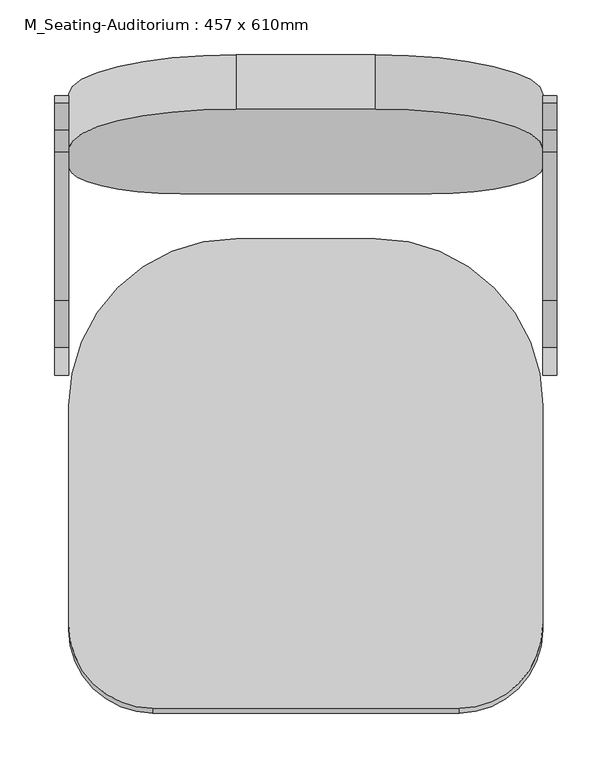
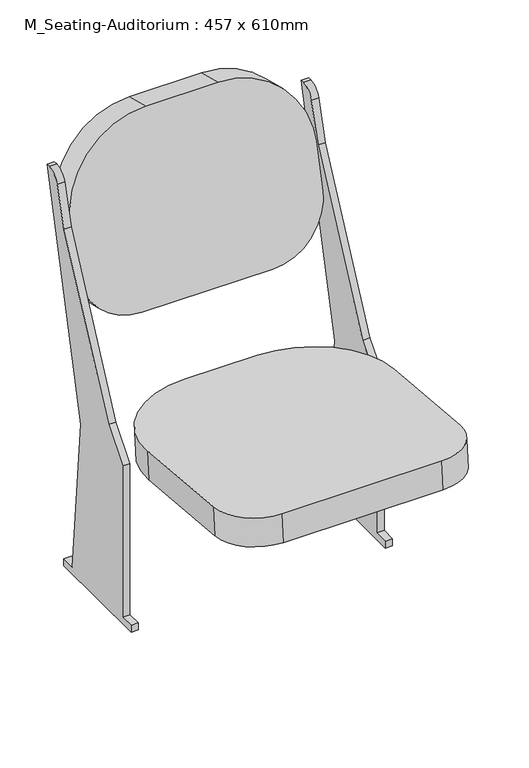
"""IFC4 building model written with IfcOpenShell, lengths in millimetres: furniture geometry, M_Seating-Auditorium : 457 x 610mm."""

from ifc_helpers import new_model, si_unit, point, frame, frame_2d, origin, place, context, project, spatial, polyline, circle_curve, trimmed, segment, composite_curve, outline, extrude, source, transform, mapped, element, save


def m_seating_auditorium_457_x_610mm_4fdbbe14(model_context):
    return source(origin(), model_context, "Body", "SweptSolid", [
        extrude(outline(composite_curve([segment(polyline([(13.3245902, 12.7), (13.3245902, 0.0), (-189.8754098, 0.0), (-189.8754098, 12.7), (-164.4754098, 12.7), (-164.4754098, 292.1), (-121.8491486, 342.9), (13.3245902, 622.3), (33.4611378, 692.7779166)]), True, "CONTINUOUS"), segment(trimmed(circle_curve(frame_2d((57.883846, 685.8)), 25.4), [point((33.4611378, 692.7779166))], [point((57.883846, 711.2))], False, "CARTESIAN"), True, "CONTINUOUS"), segment(polyline([(57.883846, 711.2), (64.1245902, 711.2), (-37.4754098, 292.1), (-12.0754098, 12.7), (13.3245902, 12.7)]), True, "CONTINUOUS")], self_intersect=False)), frame((376.6278689, 0.0, 0.0), z_axis=(1.0, 0.0, 0.0), x_axis=(0.0, 1.0, 0.0)), (0.0, 0.0, 1.0), 12.7),
        extrude(outline(composite_curve([segment(polyline([(13.3245902, 0.0), (-189.8754098, 0.0), (-189.8754098, 12.7), (-164.4754098, 12.7), (-164.4754098, 292.1), (-121.8491486, 342.9), (13.3245902, 622.3), (33.4611378, 692.7779166)]), True, "CONTINUOUS"), segment(trimmed(circle_curve(frame_2d((57.883846, 685.8)), 25.4), [point((33.4611378, 692.7779166))], [point((57.883846, 711.2))], False, "CARTESIAN"), True, "CONTINUOUS"), segment(polyline([(57.883846, 711.2), (64.1245902, 711.2), (-37.4754098, 292.1), (-12.0754098, 12.7), (13.3245902, 12.7), (13.3245902, 0.0)]), True, "CONTINUOUS")], self_intersect=False)), frame((-67.8721311, 0.0, 0.0), z_axis=(1.0, 0.0, 0.0), x_axis=(0.0, 1.0, 0.0)), (0.0, 0.0, 1.0), 12.7),
        extrude(outline(composite_curve([segment(polyline([(0.0, 0.0), (-279.4, 0.0)]), True, "CONTINUOUS"), segment(trimmed(circle_curve(frame_2d((-279.4, 76.2)), 76.2), [point((-279.4, 0.0))], [point((-355.6, 76.2))], False, "CARTESIAN"), True, "CONTINUOUS"), segment(polyline([(-355.6, 76.2), (-355.6, 276.4123505)]), True, "CONTINUOUS"), segment(trimmed(circle_curve(frame_2d((-203.2, 276.4123505)), 152.4), [point((-355.6, 276.4123505))], [point((-203.2, 428.8123506))], False, "CARTESIAN"), True, "CONTINUOUS"), segment(polyline([(-203.2, 428.8123506), (-76.2, 428.8123506)]), True, "CONTINUOUS"), segment(trimmed(circle_curve(frame_2d((-76.2, 276.4123505)), 152.4), [point((-76.2, 428.8123506))], [point((76.2, 276.4123505))], False, "CARTESIAN"), True, "CONTINUOUS"), segment(polyline([(76.2, 276.4123505), (76.2, 76.2)]), True, "CONTINUOUS"), segment(trimmed(circle_curve(frame_2d((0.0, 76.2)), 76.2), [point((76.2, 76.2))], [point((0.0, 0.0))], False, "CARTESIAN"), True, "CONTINUOUS")], self_intersect=False)), frame((300.4278689, -497.5245173, 321.2380213), z_axis=(0.0, 0.08715574274765496, 0.9961946980917459), x_axis=(1.0, 0.0, 0.0)), (0.0, 0.0, 1.0), 50.8),
        extrude(outline(composite_curve([segment(trimmed(circle_curve(frame_2d((0.0, 152.4)), 152.4), [point((0.0, 0.0))], [point((-152.4, 152.4))], False, "CARTESIAN"), True, "CONTINUOUS"), segment(polyline([(-152.4, 152.4), (-152.4, 224.0588601)]), True, "CONTINUOUS"), segment(trimmed(circle_curve(frame_2d((-50.8, 224.0588601)), 101.6), [point((-152.4, 224.0588601))], [point((-50.8, 325.6588601))], False, "CARTESIAN"), True, "CONTINUOUS"), segment(polyline([(-50.8, 325.6588601), (177.8, 325.6588601)]), True, "CONTINUOUS"), segment(trimmed(circle_curve(frame_2d((177.8, 224.0588601)), 101.6), [point((177.8, 325.6588601))], [point((279.4, 224.0588601))], False, "CARTESIAN"), True, "CONTINUOUS"), segment(polyline([(279.4, 224.0588601), (279.4, 152.4)]), True, "CONTINUOUS"), segment(trimmed(circle_curve(frame_2d((127.0, 152.4)), 152.4), [point((279.4, 152.4))], [point((127.0, 0.0))], False, "CARTESIAN"), True, "CONTINUOUS"), segment(polyline([(127.0, 0.0), (0.0, 0.0)]), True, "CONTINUOUS")], self_intersect=False)), frame((224.2278689, 101.3396919, 755.9484479), z_axis=(0.0, -0.9717404775047361, 0.23605178325712217), x_axis=(-1.0, 0.0, 0.0)), (0.0, 0.0, 1.0), 50.8),
    ])


if __name__ == "__main__":
    model = new_model("IFC4")
    model_context = context("Model", 3, world=origin())
    ifc_project = project(units=[si_unit("LENGTHUNIT", "METRE", prefix="MILLI")], contexts=[model_context])
    site = spatial("IfcSite", under=ifc_project)
    building = spatial("IfcBuilding", under=site)
    placement = place(None, origin())
    m_seating_auditorium_457_x_610mm_shape = m_seating_auditorium_457_x_610mm_4fdbbe14(model_context)
    element("IfcFurniture", 1, ObjectType="M_Seating-Auditorium : 457 x 610mm", at=placement, inside=building, context=model_context, shape_type="MappedRepresentation", body=[
        mapped(m_seating_auditorium_457_x_610mm_shape, transform((0.0, 0.0, 0.0), x_axis=(1.0, 0.0, 0.0), y_axis=(0.0, 1.0, 0.0), z_axis=(0.0, 0.0, 1.0))),
    ])
    save(model, "model.ifc")

# Revit data of these elements
# Type "M_Seating-Auditorium : 457 x 610mm"
#   Seat/Back Material = Linen, Beige
#   Frame Material = Steel, Paint Finish, Dark Gray, Matte
#   Default Elevation = 0
# Element 1 (IfcFurniture, "M_Seating-Auditorium : 457 x 610mm")
#   Materials on its faces: "Steel, Paint Finish, Dark Gray, Matte", "Linen, Beige"
# Materials
#   "Linen, Beige": class "Textile", colour RGB 249 239 230, transparency 0, Description = "Linen, beige", Cost = 0
#   "Steel, Paint Finish, Dark Gray, Matte": class "Metal", colour RGB 0 0 0, transparency 0, Description = "Steel, paint finish, dark gray, matte", Cost = 0
